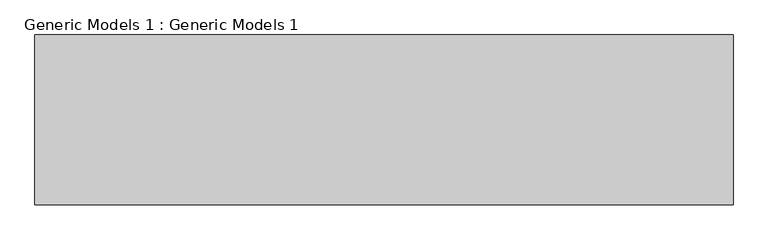
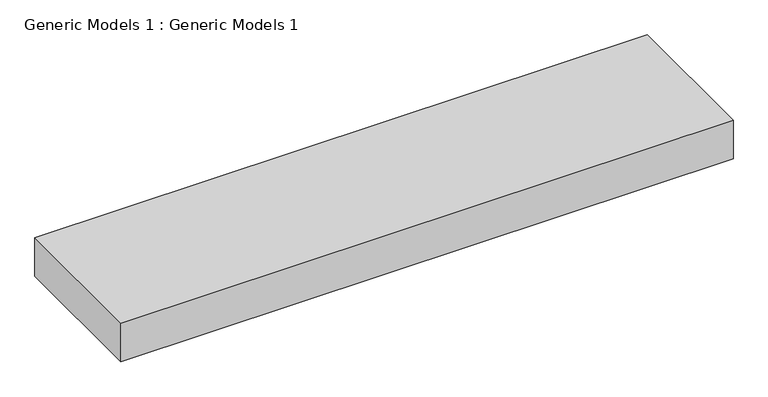
"""IFC4 building model written with IfcOpenShell, lengths in millimetres: proxy geometry, Generic Models 1 : Generic Models 1."""

from ifc_helpers import new_model, si_unit, origin, origin_with_axes, place, context, project, spatial, polyline, outline, extrude, source, transform, mapped, element, save


def generic_models_1_generic_models_1_2766a2ed(model_context):
    return source(origin(), model_context, "Body", "SweptSolid", [
        extrude(outline(polyline([(-7984.0518575, -15154.7378384), (-7984.0518575, -16266.353918), (-12556.0518575, -16266.353918), (-12556.0518575, -15154.7378384), (-7984.0518575, -15154.7378384)])), origin_with_axes(), (0.0, 0.0, 1.0), 304.8),
    ])


if __name__ == "__main__":
    model = new_model("IFC4")
    model_context = context("Model", 3, world=origin())
    ifc_project = project(units=[si_unit("LENGTHUNIT", "METRE", prefix="MILLI")], contexts=[model_context])
    site = spatial("IfcSite", under=ifc_project)
    building = spatial("IfcBuilding", under=site)
    placement = place(None, origin())
    generic_models_1_generic_models_1_shape = generic_models_1_generic_models_1_2766a2ed(model_context)
    element("IfcBuildingElementProxy", 1, Name="Generic Models 1 : Generic Models 1", ObjectType="Generic Models 1 : Generic Models 1", at=placement, inside=building, context=model_context, shape_type="MappedRepresentation", body=[
        mapped(generic_models_1_generic_models_1_shape, transform((0.0, 0.0, 0.0), x_axis=(1.0, 0.0, 0.0), y_axis=(0.0, 1.0, 0.0), z_axis=(0.0, 0.0, 1.0))),
    ])
    save(model, "model.ifc")
